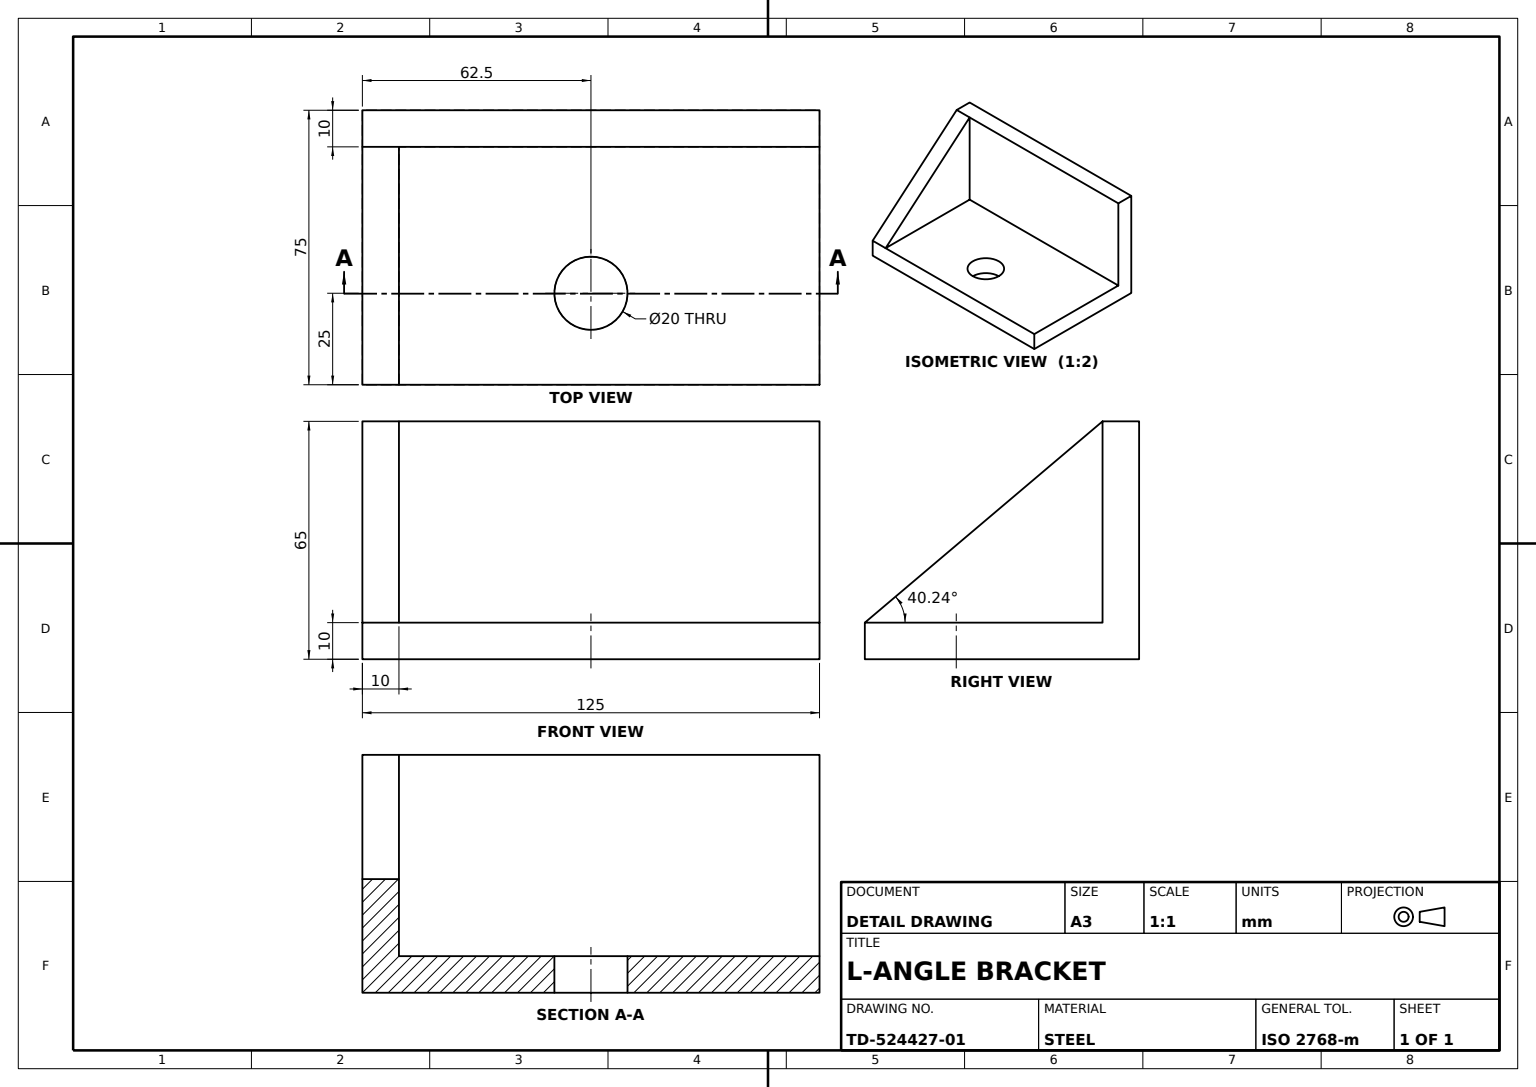
SolidWorks part; units mm, degrees
material "Plain Carbon Steel"
ref_plane "Front Plane" through (0, 0, 0) normal (0, 0, 1) x (1, 0, 0)
ref_plane "Top Plane" through (0, 0, 0) normal (0, 1, 0) x (1, 0, 0)
ref_plane "Right Plane" through (0, 0, 0) normal (1, 0, 0) x (0, 0, -1)
sketch "Base Plate Profile" plane through (0, 0, 0) normal (0, 0, 1) x (1, 0, 0)
  line L1 (0, 0) -> (125, 0)
  line L2 (0, 0) -> (0, 10)
  line L3 (0, 10) -> (125, 10)
  line L4 (125, 0) -> (125, 10)
  dimension "D1" = 125
  dimension "D2" = 10
extrude "Base Plate" add sketch "Base Plate Profile" along normal blind 75
sketch "Back Wall Profile" plane through (0, 10, 0) normal (0, 1, 0) x (1, 0, 0)
  line L0 (125, -75) -> (125, 0) construction
  line L1 (0, 0) -> (125, 0)
  line L2 (0, 0) -> (0, -10)
  line L3 (0, -10) -> (125, -10)
  line L4 (125, 0) -> (125, -10)
  dimension "D1" = 10
extrude "Back Wall" add sketch "Back Wall Profile" along normal blind 55
sketch "End Wall Profile" plane through (0, 10, 0) normal (0, 1, 0) x (1, 0, 0)
  line L0 (0, -10) -> (125, -10) construction
  line L1 (0, -75) -> (10, -75)
  line L2 (0, -75) -> (0, -10)
  line L3 (0, -10) -> (10, -10)
  line L4 (10, -75) -> (10, -10)
  dimension "D1" = 10
extrude "End Wall" add sketch "End Wall Profile" along normal blind 55
sketch "Gusset Trim Profile" plane through (10, 0, 0) normal (1, 0, 0) x (0, 0, -1)
  line L0 (-10, 65) -> (-75, 10)
  line L1 (-75, 10) -> (-75, 65)
  line L2 (-75, 65) -> (-10, 65)
extrude "Gusset Trim Cut" cut sketch "Gusset Trim Profile" against normal blind 55
sketch "Base Hole Ø20 Sketch" plane through (0, 10, 0) normal (0, 1, 0) x (1, 0, 0)
  line L0 (125, -75) -> (125, -10) construction
  line L1 (125, -75) -> (10, -75) construction
  circle A0 centre (62.5, -50) radius 10
  dimension "D1" = 20
  dimension "D2" = 62.5
  dimension "D3" = 25
extrude "Base Hole Ø20" cut sketch "Base Hole Ø20 Sketch" against normal blind 55
